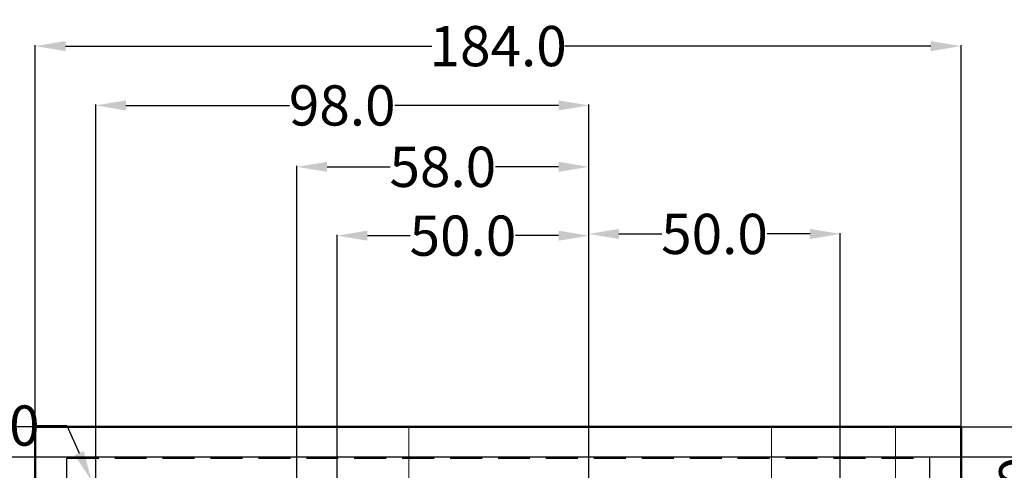
# Model space of a CAD drawing. Units: inches. Extents: x 11765 to 12471, y 10149 to 10793.
# Tile 6 of 8: x 11880 to 12076, y 10704 to 10793. Entities that reach past the tile are written whole.
import ezdxf

# ---------------------------------------------------------------- set-up
doc = ezdxf.new("R2010")
doc.units = ezdxf.units.IN
doc.header["$MEASUREMENT"] = 0
doc.linetypes.add('CENTER', pattern=[50.8, 31.75, -6.35, 6.35, -6.35])
doc.linetypes.add('HIDDEN', pattern=[9.525, 6.35, -3.175])
for name, color, linetype, lineweight in [('M-CNTR', 30, 'CENTER', 18), ('M-DIMS', 2, 'Continuous', 25), ('M-HIDN', 41, 'HIDDEN', 25), ('M-OUTL', 7, 'Continuous', 50)]:
    doc.layers.add(name, color=color, linetype=linetype, lineweight=lineweight)
doc.styles.get("Standard").update_dxf_attribs({"font": 'arial.ttf'})
doc.dimstyles.get("Standard").update_dxf_attribs({"dimtxt": 8, "dimasz": 6, "dimexe": 0.18, "dimexo": 0.0625, "dimgap": 0.09, "dimtad": 0, "dimtoh": 1, "dimdec": 1, "dimzin": 0, "dimdsep": 46, "dimtxsty": 'Standard', "dimcen": 0.09, "dimadec": 0, "dimazin": 0, "dimtfac": 1, "dimtdec": 1, "dimtofl": 0, "dimtmove": 0, "dimatfit": 3, "dimfxl": 1, "dimtolj": 1, "dimtzin": 0, "dimarcsym": 0})

# ---------------------------------------------------------------- blocks, each defined once
blk = doc.blocks.new('*D1')
at = {"layer": 'Defpoints', "color": 0, "transparency": 16777216}
for p in [(12066.91, 10787.84), (11882.91, 10712.15), (12066.91, 10712.15)]:
    blk.add_point(p, dxfattribs=at)
at = {"layer": 'M-DIMS', "color": 0, "lineweight": -2, "transparency": 16777216}
for p, q in [((11882.91, 10712.21), (11882.91, 10788.02)), ((11888.91, 10787.84), (11961.71, 10787.84)), ((12060.91, 10787.84), (11988.11, 10787.84)), ((12066.91, 10712.21), (12066.91, 10788.02))]:
    blk.add_line(p, q, dxfattribs=at)
at = {"layer": 'M-DIMS', "color": 0, "transparency": 16777216}
for points in [[(11888.91, 10788.84), (11888.91, 10786.84), (11882.91, 10787.84)], [(12060.91, 10788.84), (12060.91, 10786.84), (12066.91, 10787.84)]]:
    blk.add_solid(points, dxfattribs=at)
at = {"layer": 'M-DIMS', "color": 0, "transparency": 16777216, "insert": (11974.91, 10787.84), "char_height": 8, "attachment_point": 5}
blk.add_mtext('\\A1;184.0', dxfattribs=at)
blk = doc.blocks.new('*D2')
at = {"layer": 'Defpoints', "color": 0, "transparency": 16777216}
for p in [(11894.91, 10776.05), (11992.91, 10712.15), (11894.91, 10699.65)]:
    blk.add_point(p, dxfattribs=at)
at = {"layer": 'M-DIMS', "color": 0, "lineweight": -2, "transparency": 16777216}
for p, q in [((11894.91, 10699.71), (11894.91, 10776.23)), ((11900.91, 10776.05), (11933.45, 10776.05)), ((11986.91, 10776.05), (11954.38, 10776.05)), ((11992.91, 10712.21), (11992.91, 10776.23))]:
    blk.add_line(p, q, dxfattribs=at)
at = {"layer": 'M-DIMS', "color": 0, "transparency": 16777216}
for points in [[(11900.91, 10777.05), (11900.91, 10775.05), (11894.91, 10776.05)], [(11986.91, 10777.05), (11986.91, 10775.05), (11992.91, 10776.05)]]:
    blk.add_solid(points, dxfattribs=at)
at = {"layer": 'M-DIMS', "color": 0, "transparency": 16777216, "insert": (11943.91, 10776.05), "char_height": 8, "attachment_point": 5}
blk.add_mtext('\\A1;98.0', dxfattribs=at)
blk = doc.blocks.new('*D3')
at = {"layer": 'Defpoints', "color": 0, "transparency": 16777216}
for p in [(11992.91, 10763.84), (11992.91, 10699.65), (11934.91, 10654.29)]:
    blk.add_point(p, dxfattribs=at)
at = {"layer": 'M-DIMS', "color": 0, "lineweight": -2, "transparency": 16777216}
for p, q in [((11934.91, 10654.35), (11934.91, 10764.02)), ((11940.91, 10763.84), (11953.45, 10763.84)), ((11986.91, 10763.84), (11974.38, 10763.84)), ((11992.91, 10699.71), (11992.91, 10764.02))]:
    blk.add_line(p, q, dxfattribs=at)
at = {"layer": 'M-DIMS', "color": 0, "transparency": 16777216}
for points in [[(11940.91, 10764.84), (11940.91, 10762.84), (11934.91, 10763.84)], [(11986.91, 10764.84), (11986.91, 10762.84), (11992.91, 10763.84)]]:
    blk.add_solid(points, dxfattribs=at)
at = {"layer": 'M-DIMS', "color": 0, "transparency": 16777216, "insert": (11963.91, 10763.84), "char_height": 8, "attachment_point": 5}
blk.add_mtext('\\A1;58.0', dxfattribs=at)
blk = doc.blocks.new('*D4')
at = {"layer": 'Defpoints', "color": 0, "transparency": 16777216}
for p in [(11992.91, 10750.16), (11992.91, 10699.65), (11942.91, 10630.15)]:
    blk.add_point(p, dxfattribs=at)
at = {"layer": 'M-DIMS', "color": 0, "lineweight": -2, "transparency": 16777216}
for p, q in [((11942.91, 10630.21), (11942.91, 10750.34)), ((11948.91, 10750.16), (11957.45, 10750.16)), ((11986.91, 10750.16), (11978.38, 10750.16)), ((11992.91, 10699.71), (11992.91, 10750.34))]:
    blk.add_line(p, q, dxfattribs=at)
at = {"layer": 'M-DIMS', "color": 0, "transparency": 16777216}
for points in [[(11948.91, 10751.16), (11948.91, 10749.16), (11942.91, 10750.16)], [(11986.91, 10751.16), (11986.91, 10749.16), (11992.91, 10750.16)]]:
    blk.add_solid(points, dxfattribs=at)
at = {"layer": 'M-DIMS', "color": 0, "transparency": 16777216, "insert": (11967.91, 10750.16), "char_height": 8, "attachment_point": 5}
blk.add_mtext('\\A1;50.0', dxfattribs=at)
blk = doc.blocks.new('*D5')
at = {"layer": 'Defpoints', "color": 0, "transparency": 16777216}
for p in [(11992.91, 10750.5), (11992.91, 10699.65), (12042.91, 10642.79)]:
    blk.add_point(p, dxfattribs=at)
at = {"layer": 'M-DIMS', "color": 0, "lineweight": -2, "transparency": 16777216}
for p, q in [((11992.91, 10699.71), (11992.91, 10750.68)), ((12042.91, 10642.86), (12042.91, 10750.68)), ((11998.91, 10750.5), (12007.45, 10750.5)), ((12036.91, 10750.5), (12028.38, 10750.5))]:
    blk.add_line(p, q, dxfattribs=at)
at = {"layer": 'M-DIMS', "color": 0, "transparency": 16777216}
for points in [[(11998.91, 10751.5), (11998.91, 10749.5), (11992.91, 10750.5)], [(12036.91, 10751.5), (12036.91, 10749.5), (12042.91, 10750.5)]]:
    blk.add_solid(points, dxfattribs=at)
at = {"layer": 'M-DIMS', "color": 0, "transparency": 16777216, "insert": (12017.91, 10750.5), "char_height": 8, "attachment_point": 5}
blk.add_mtext('\\A1;50.0', dxfattribs=at)
blk = doc.blocks.new('*D6')
at = {"layer": 'Defpoints', "color": 0, "transparency": 16777216}
for p in [(11882.91, 10712.15), (11769.87, 10237.15), (11917.55, 10237.15)]:
    blk.add_point(p, dxfattribs=at)
at = {"layer": 'M-DIMS', "color": 0, "lineweight": -2, "transparency": 16777216}
for p, q in [((11882.85, 10712.15), (11769.69, 10712.15)), ((11769.87, 10706.15), (11769.87, 10488.38)), ((11769.87, 10243.15), (11769.87, 10460.91)), ((11917.49, 10237.15), (11769.69, 10237.15))]:
    blk.add_line(p, q, dxfattribs=at)
at = {"layer": 'M-DIMS', "color": 0, "transparency": 16777216}
for points in [[(11768.87, 10706.15), (11770.87, 10706.15), (11769.87, 10712.15)], [(11768.87, 10243.15), (11770.87, 10243.15), (11769.87, 10237.15)]]:
    blk.add_solid(points, dxfattribs=at)
at = {"layer": 'M-DIMS', "color": 0, "transparency": 16777216, "insert": (11769.87, 10474.65), "char_height": 8, "attachment_point": 5, "rotation": 90}
blk.add_mtext('\\A1;475.0', dxfattribs=at)
blk = doc.blocks.new('*D24')
at = {"layer": 'Defpoints', "color": 0, "transparency": 16777216}
for p in [(11794.92, 10712.15), (11882.91, 10712.15), (11882.91, 10592.15)]:
    blk.add_point(p, dxfattribs=at)
at = {"layer": 'M-DIMS', "color": 0, "lineweight": -2, "transparency": 16777216}
for p, q in [((11882.85, 10712.15), (11794.74, 10712.15)), ((11794.92, 10706.15), (11794.92, 10665.34)), ((11794.92, 10598.15), (11794.92, 10638.95)), ((11882.85, 10592.15), (11794.74, 10592.15))]:
    blk.add_line(p, q, dxfattribs=at)
at = {"layer": 'M-DIMS', "color": 0, "transparency": 16777216}
for points in [[(11793.92, 10706.15), (11795.92, 10706.15), (11794.92, 10712.15)], [(11793.92, 10598.15), (11795.92, 10598.15), (11794.92, 10592.15)]]:
    blk.add_solid(points, dxfattribs=at)
at = {"layer": 'M-DIMS', "color": 0, "transparency": 16777216, "insert": (11794.92, 10652.15), "char_height": 8, "attachment_point": 5, "rotation": 90}
blk.add_mtext('\\A1;120.0', dxfattribs=at)
blk = doc.blocks.new('*D28')
at = {"layer": 'Defpoints', "color": 0, "transparency": 16777216}
for p in [(12053.91, 10712.15), (12078.49, 10712.15), (12053.91, 10679.15)]:
    blk.add_point(p, dxfattribs=at)
at = {"layer": 'M-DIMS', "color": 0, "lineweight": -2, "transparency": 16777216}
for p, q in [((12078.49, 10718.15), (12078.49, 10724.15)), ((12053.97, 10712.15), (12078.67, 10712.15)), ((12053.97, 10679.15), (12078.67, 10679.15)), ((12078.49, 10673.15), (12078.49, 10667.15))]:
    blk.add_line(p, q, dxfattribs=at)
at = {"layer": 'M-DIMS', "color": 0, "transparency": 16777216}
for points in [[(12077.49, 10718.15), (12079.49, 10718.15), (12078.49, 10712.15)], [(12077.49, 10673.15), (12079.49, 10673.15), (12078.49, 10679.15)]]:
    blk.add_solid(points, dxfattribs=at)
at = {"layer": 'M-DIMS', "color": 0, "transparency": 16777216, "insert": (12078.49, 10695.65), "char_height": 8, "attachment_point": 5, "rotation": 90}
blk.add_mtext('\\A1;33.0', dxfattribs=at)
blk = doc.blocks.new('*D62')
at = {"layer": 'Defpoints', "color": 0, "transparency": 16777216}
for p in [(12379.9, 10706.15), (11848.16, 10684.29), (12385.4, 10684.29)]:
    blk.add_point(p, dxfattribs=at)
at = {"layer": 'M-DIMS', "color": 0, "lineweight": -2, "transparency": 16777216}
for p, q in [((12379.83, 10706.15), (11847.98, 10706.15)), ((11848.16, 10700.15), (11848.16, 10690.29)), ((12385.33, 10684.29), (11847.98, 10684.29)), ((11848.16, 10684.29), (11848.16, 10678.29)), ((11848.16, 10678.29), (11842.16, 10678.29))]:
    blk.add_line(p, q, dxfattribs=at)
at = {"layer": 'M-DIMS', "color": 0, "transparency": 16777216}
for points in [[(11847.16, 10700.15), (11849.16, 10700.15), (11848.16, 10706.15)], [(11847.16, 10690.29), (11849.16, 10690.29), (11848.16, 10684.29)]]:
    blk.add_solid(points, dxfattribs=at)
at = {"layer": 'M-DIMS', "color": 0, "transparency": 16777216, "insert": (11828.51, 10678.29), "char_height": 8, "attachment_point": 5}
blk.add_mtext('\\A1;21.86', dxfattribs=at)
blk = doc.blocks.new('*D83')
at = {"layer": 'Defpoints', "color": 0, "transparency": 16777216}
for p in [(11894.09, 10701.47), (11895.73, 10697.82)]:
    blk.add_point(p, dxfattribs=at)
at = {"layer": 'M-DIMS', "color": 0, "lineweight": -2, "transparency": 16777216}
for p, q in [((11883.16, 10712.41), (11889.16, 10712.41)), ((11889.16, 10712.41), (11891.62, 10706.94)), ((11894.82, 10699.65), (11895, 10699.65)), ((11894.91, 10699.56), (11894.91, 10699.74))]:
    blk.add_line(p, q, dxfattribs=at)
at = {"layer": 'M-DIMS', "color": 0, "transparency": 16777216}
blk.add_solid([(11892.53, 10707.35), (11890.71, 10706.53), (11894.09, 10701.47)], dxfattribs=at)
at = {"layer": 'M-DIMS', "color": 0, "transparency": 16777216, "insert": (11860.33, 10712.41), "char_height": 8, "attachment_point": 5}
blk.add_mtext('\\A1;13X ∅4.0', dxfattribs=at)

msp = doc.modelspace()

# ---------------------------------------------------------------- linework, layer by layer
at = {"layer": 'M-CNTR'}
for p, q in [((11942.912, 10237.146), (11942.912, 10712.146)), ((11957.122, 10237.146), (11957.122, 10712.146)), ((11992.912, 10237.146), (11992.912, 10712.146)), ((12029.232, 10237.146), (12029.232, 10712.146)), ((12042.912, 10504.146), (12042.912, 10712.146)), ((12053.912, 10237.146), (12053.912, 10712.146))]:
    msp.add_line(p, q, dxfattribs=at)
at = {"layer": 'M-HIDN'}
msp.add_lwpolyline([(12060.662, 10705.896), (12060.662, 10515.896), (12096.662, 10515.896), (12096.662, 10263.352), (12062.096, 10243.396), (11923.728, 10243.396), (11889.162, 10263.352), (11889.162, 10705.896)], close=True, dxfattribs=at)
at = {"layer": 'M-OUTL'}
for p, q in [((12066.912, 10712.146), (11882.912, 10712.146)), ((11882.912, 10712.146), (11882.912, 10257.146)), ((12066.912, 10522.146), (12066.912, 10712.146))]:
    msp.add_line(p, q, dxfattribs=at)

# ---------------------------------------------------------------- dimensions: what is measured, and where the dimension line sits
at = {"layer": 'M-DIMS'}
for base, p1, p2, picture, middle in [((12066.912, 10787.841), (11882.912, 10712.146), (12066.912, 10712.146), '*D1', (11974.912, 10787.841)), ((11894.912, 10776.05), (11992.912, 10712.146), (11894.912, 10699.646), '*D2', (11943.912, 10776.05)), ((11992.912, 10763.836), (11934.912, 10654.286), (11992.912, 10699.646), '*D3', (11963.912, 10763.836)), ((11992.912, 10750.16), (11942.912, 10630.146), (11992.912, 10699.646), '*D4', (11967.912, 10750.16)), ((11992.912, 10750.499), (12042.912, 10642.793), (11992.912, 10699.646), '*D5', (12017.912, 10750.499))]:
    dim = msp.add_linear_dim(base=base, p1=p1, p2=p2, dimstyle='Standard', override={"dimclrd": 0, "dimclre": 0, "dimclrt": 0}, dxfattribs=at)
    dim.commit()
    dim.dimension.update_dxf_attribs({"geometry": picture, "text_midpoint": middle})
dim = msp.add_diameter_dim_2p(p1=(11895.734, 10697.822), p2=(11894.09, 10701.469), text='13X <>', dimstyle='Standard', override={"dimdec": 1, "dimlfac": 1, "dimrnd": 0, "dimzin": 0, "dimdsep": 46, "dimlunit": 2}, dxfattribs=at)
dim.commit()
dim.dimension.update_dxf_attribs({"geometry": '*D83', "text_midpoint": (11860.332, 10712.407), "dimtype": 163})
for base, p1, p2, override, picture, middle in [((12078.487, 10712.146), (12053.912, 10679.146), (12053.912, 10712.146), {"dimclrd": 0, "dimclre": 0, "dimclrt": 0}, '*D28', (12078.487, 10695.646)), ((11769.869, 10237.146), (11882.912, 10712.146), (11917.553, 10237.146), {"dimclrd": 0, "dimclre": 0, "dimclrt": 0}, '*D6', (11769.869, 10474.646)), ((11794.917, 10712.146), (11882.912, 10592.146), (11882.912, 10712.146), {"dimclrd": 0, "dimclre": 0, "dimclrt": 0}, '*D24', (11794.917, 10652.146)), ((11848.162, 10684.286), (12379.896, 10706.146), (12385.396, 10684.286), {"dimdec": 2, "dimlfac": 1, "dimrnd": 0, "dimzin": 0, "dimdsep": 46, "dimlunit": 2}, '*D62', (11828.509, 10678.286))]:
    dim = msp.add_linear_dim(base=base, p1=p1, p2=p2, angle=90, dimstyle='Standard', override=override, dxfattribs=at)
    dim.commit()
    dim.dimension.update_dxf_attribs({"geometry": picture, "text_midpoint": middle})

doc.saveas('drawing.dxf')
